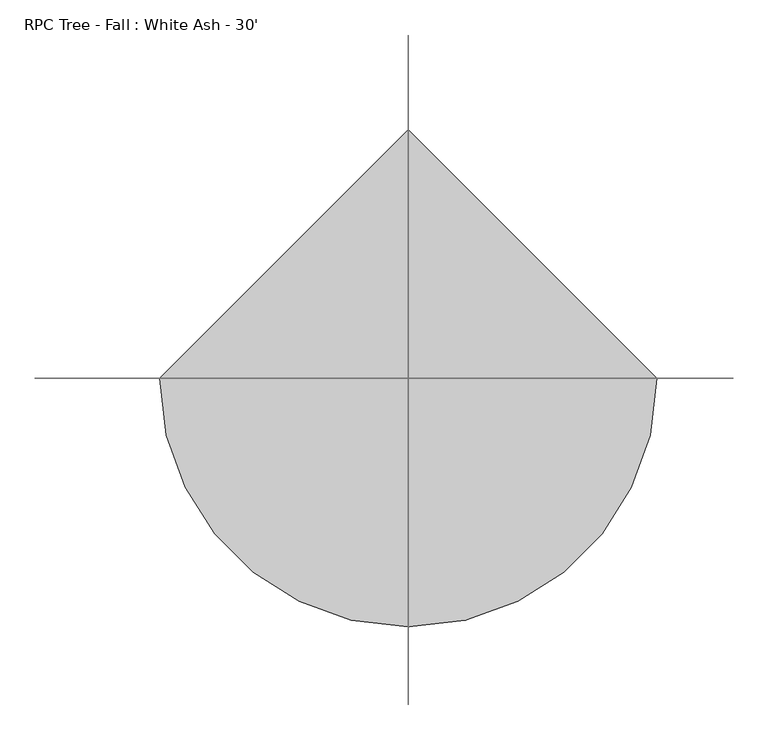
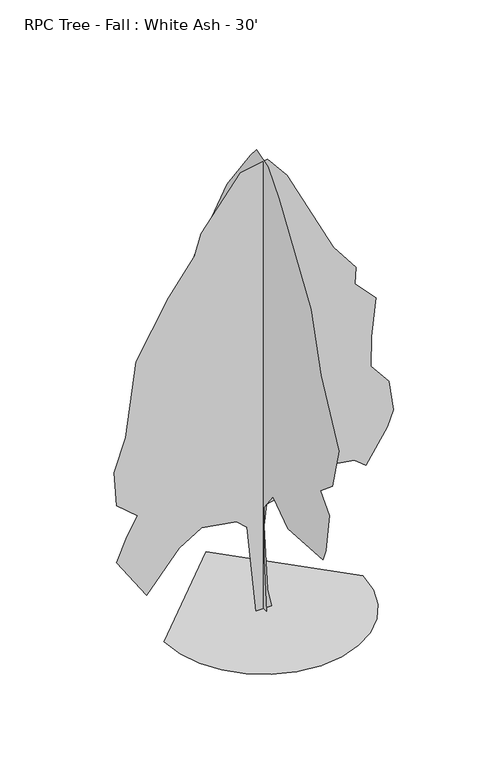
"""IFC4 building model written with IfcOpenShell, lengths in millimetres: geographic element geometry, RPC Tree - Fall : White Ash - 30'."""

from ifc_helpers import new_model, si_unit, origin, place, context, project, spatial, triangles, source, transform, mapped, element, save


def rpc_tree_fall_white_ash_30_ca342e74(model_context):
    return source(origin(), model_context, "Body", "Tessellation", [
        triangles([(-1903.1117432, 0.0, 0.0), (-1852.7994072, -436.0675326, 0.0), (-1709.5128044, -836.5267736, 0.0), (-1484.7201302, -1189.902079, 0.0), (-1189.902079, -1484.7201302, 0.0), (-836.5243029, -1709.5103336, 0.0), (-436.0675326, -1852.7994072, 0.0), (8.32e-05, -1903.1117432, 0.0), (436.0675326, -1852.7994072, 0.0), (836.5267736, -1709.5128044, 0.0), (1189.902079, -1484.7201302, 0.0), (1484.7201302, -1189.902079, 0.0), (1709.5103336, -836.5243029, 0.0), (1852.7994072, -436.0675326, 0.0), (1903.1117432, 0.0001664, 0.0), (-0.0002496, 1903.1117432, 0.0), (-6.4e-06, -107.924944, 0.0613456), (2.91e-05, -19.1547901, 1015.9932175), (6.03e-05, -22.4623803, 2068.4709812), (5.39e-05, -325.6028727, 2458.2394867), (1.45e-05, -807.5987429, 2100.6274487), (-5.27e-05, -1977.9757782, 2188.0796688), (-5.09e-05, -2067.0104599, 2427.1421116), (-3.51e-05, -2191.3969082, 3204.5680595), (-7.8e-06, -1895.979475, 3531.0600494), (-2.12e-05, -2284.6861267, 3857.5773285), (-9.2e-06, -2502.3617935, 4697.2004974), (6.13e-05, -1911.529398, 5878.860347), (0.0001153, -1572.9038464, 7015.6124725), (0.0002258, -512.181237, 8599.811705), (0.0002601, -154.5713246, 9035.1682709), (0.0002865, 234.1363626, 9144.0075577), (0.0002913, 433.9238045, 8906.4918228), (0.0003064, 1213.6790434, 7853.5084213), (0.0003087, 2239.8677868, 5877.6918137), (0.0003058, 2576.679641, 5106.6993393), (0.0002851, 2628.5718224, 4308.4785851), (0.0002675, 2473.0932312, 4028.6209579), (0.000235, 2395.3514648, 3095.7290634), (0.0002321, 2555.4707611, 2675.9174789), (0.0001966, 2115.4813385, 2364.9501228), (0.0001827, 2177.675798, 1774.1152565), (0.0001544, 1919.8426987, 1341.3319347), (0.0001354, 1726.7746868, 1089.9885555), (9.37e-05, 700.5858707, 1743.0180267), (9e-05, 514.0075064, 1991.7909233), (7.64e-05, 345.4377448, 1871.6004398), (4.67e-05, 163.0671178, 1239.2314808), (5.8e-06, 97.9767685, 0.0613703), (-139.7232302, 6.1e-06, 0.0682885), (-310.5051023, -0.0001955, 1753.6784225), (-510.5150233, -0.0002089, 1939.8629883), (-1184.5807468, -0.0001927, 2050.8713287), (-1618.5299858, -0.0001419, 1783.914513), (-2238.7425648, -2.84e-05, 1058.8988834), (-2814.0427689, -0.0001052, 1914.0565693), (-2611.9094673, -0.0001696, 2380.5051327), (-2409.7761658, -0.0002192, 2722.5774216), (-2814.0427689, -0.0002423, 3064.6393913), (-2860.6774223, -0.0003218, 3748.7636215), (-2642.9991394, -0.0004074, 4386.2279091), (-2440.8707794, -0.0005904, 5847.7703842), (-1817.4934227, -0.0007464, 6927.6777237), (-1321.3953609, -0.0008469, 7589.1960663), (-1197.0064419, -0.0009024, 8008.9820709), (-435.1404453, -0.0010506, 8972.9889267), (77.9529181, -0.0010842, 9066.2832321), (451.1119632, -0.0010468, 8615.3822662), (1343.785564, -0.0008745, 6842.8672028), (1771.7911251, -0.0008273, 6290.4422012), (1757.1683258, -0.0007869, 5956.609671), (2157.6860298, -0.0007547, 5539.8967346), (2072.4358555, -0.0006605, 4780.5631416), (2056.3779694, -0.0005886, 4183.7135262), (2399.5679226, -0.0005536, 3764.3083122), (2487.9397087, -0.0004852, 3157.9084076), (2379.1005672, -0.0004434, 2846.9613991), (1961.5166084, -0.0003491, 2209.4741478), (1741.621019, -0.0003618, 2396.0524395), (1104.141398, -0.0003453, 2491.7598244), (637.6903639, -0.0003117, 2380.5051327), (353.060281, -0.0002734, 2163.9953831), (54.4347815, -0.000252, 2094.0056145), (14.3638898, -0.0002002, 1674.2703335), (82.551847, -4.67e-05, 361.775047), (152.5283897, -6.7e-06, 0.0682758)], [[15, 16, 1], [14, 15, 1], [14, 1, 2], [13, 14, 2], [13, 2, 3], [13, 3, 4], [12, 13, 4], [11, 12, 4], [11, 4, 5], [11, 5, 6], [11, 6, 7], [11, 7, 8], [11, 8, 9], [11, 9, 10], [48, 49, 17], [48, 17, 18], [48, 18, 19], [47, 48, 19], [43, 44, 45], [42, 43, 45], [41, 42, 45], [41, 45, 46], [39, 40, 41], [31, 32, 33], [21, 22, 23], [21, 23, 24], [21, 24, 25], [20, 21, 25], [46, 47, 19], [30, 31, 33], [30, 33, 34], [29, 30, 34], [29, 34, 35], [28, 29, 35], [28, 35, 36], [28, 36, 37], [28, 37, 38], [27, 28, 38], [26, 27, 38], [25, 26, 38], [20, 25, 38], [20, 38, 39], [20, 39, 41], [20, 41, 46], [20, 46, 19], [85, 86, 50], [85, 50, 51], [84, 85, 51], [54, 55, 56], [54, 56, 57], [77, 78, 79], [83, 84, 51], [83, 51, 52], [54, 57, 58], [53, 54, 58], [66, 67, 68], [65, 66, 68], [65, 68, 69], [64, 65, 69], [63, 64, 69], [62, 63, 69], [61, 62, 69], [61, 69, 70], [61, 70, 71], [61, 71, 72], [61, 72, 73], [61, 73, 74], [60, 61, 74], [59, 60, 74], [58, 59, 74], [53, 58, 74], [52, 53, 74], [83, 52, 74], [82, 83, 74], [81, 82, 74], [80, 81, 74], [80, 74, 75], [79, 80, 75], [77, 79, 75], [77, 75, 76]], closed=False),
    ])


if __name__ == "__main__":
    model = new_model("IFC4")
    model_context = context("Model", 3, world=origin())
    ifc_project = project(units=[si_unit("LENGTHUNIT", "METRE", prefix="MILLI")], contexts=[model_context])
    site = spatial("IfcSite", under=ifc_project)
    building = spatial("IfcBuilding", under=site)
    placement = place(None, origin())
    rpc_tree_fall_white_ash_30_shape = rpc_tree_fall_white_ash_30_ca342e74(model_context)
    element("IfcGeographicElement", 1, ObjectType="RPC Tree - Fall : White Ash - 30'", at=placement, inside=building, context=model_context, shape_type="MappedRepresentation", body=[
        mapped(rpc_tree_fall_white_ash_30_shape, transform((0.0, 0.0, 0.0), x_axis=(1.0, 0.0, 0.0), y_axis=(0.0, 1.0, 0.0), z_axis=(0.0, 0.0, 1.0))),
    ])
    save(model, "model.ifc")

# Revit data of these elements
# Type "RPC Tree - Fall : White Ash - 30'"
#   built-in parameter 1005198 = "{2, 15},{39, RPC-16-G1AF-G8PX-CFC7-2000-ST1L-LVER-AU},{1, 0},{1, 0},{2, 13},{1, 8},{5, Color},{1, 0},{1, 0},{3, 0.8},{3, 0.8},{3, 0.8},{1, 8},{7, BBoxMin},{1, 0},{1, 0},{1, 0},{1, 0},{1, 0},{1, 8},{7, BBoxMax},{1, 0},{1, 0},{1, 0},{1, 0},{1, 0},{2, 11},{9, RPCTypeId},{1, 0},{1, 0},{39, RPC-16-G1AF-G8PX-CFC7-2000-ST1L-LVER-AU},{1, 6},{14, RPCPlantHeight},{1, 0},{1, 0},{2, 30},{2, 11},{7, keyword},{1, 0},{1, 0},{39, :RPCs:Fall Trees [General]:Geometry:RPC},{2, 11},{8, category},{1, 0},{1, 0},{20, Fall Trees [General]},{2, 11},{12, LocalizedUID},{1, 0},{1, 0},{16, White Ash [Fall]},{2, 14},{6, Height},{1, 0},{1, 0},{2, 30},{1, 2},{16, Cast Reflections},{1, 0},{1, 0},{1, 0},{1, 2},{12, Cast Shadows},{1, 0},{1, 0},{1, 1},{1, 2},{9, Lock View},{1, 0},{1, 0},{1, 0},{1, 4},{5, ViewC},{1, 0},{1, 0},{1, 0},{21, assetlibrary_base.fbx},{1, 5},"
#   built-in parameter 1005195 = "RPC-16-G1AF-G8PX-CFC7-2000-ST1L-LVER-AU"
#   Type Comments = "White Ash"
#   Assembly Code = "G2050500"
#   Height = 30' - 0"
#   Default Elevation = 0
